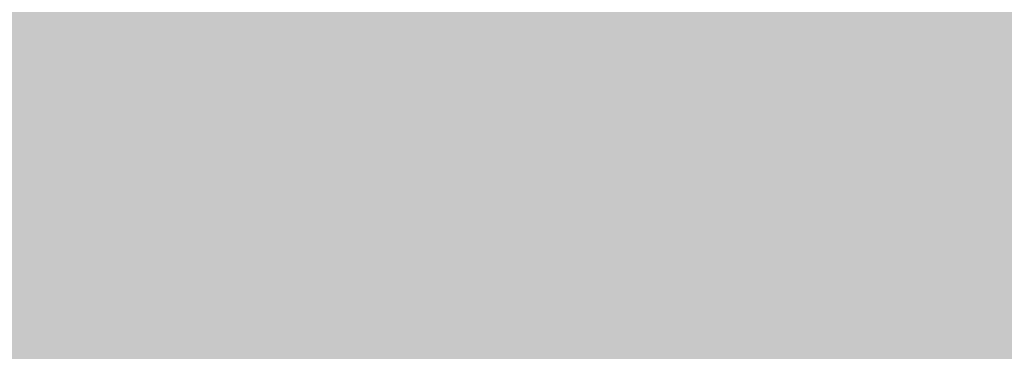
# Model space of a CAD drawing. Units: feet. Extents: x 3168 to 4724, y 827 to 1477.
# Tile 138 of 256: x 3301.129829 to 3301.134076, y 1099.01485 to 1099.016281. Entities that reach past the tile are written whole.
import ezdxf

# ---------------------------------------------------------------- set-up
doc = ezdxf.new("R2010")
doc.units = ezdxf.units.FT
doc.layers.add('A-ELEV', color=7, linetype='Continuous', lineweight=35)
doc.layers.add('A-ELEV-PATT', color=8, linetype='Continuous', lineweight=13)

msp = doc.modelspace()

# ---------------------------------------------------------------- hatches: boundary and pattern name
at = {"layer": 'A-ELEV-PATT'}
h = msp.add_hatch(color=256, dxfattribs=at)
h.dxf.hatch_style = 1
edge = h.paths.add_edge_path()
edge.add_ellipse((3552.9057615, 979.2201412), major_axis=(36.7449243, 0), ratio=0.4848484848, start_angle=0, end_angle=360)
edge = h.paths.add_edge_path()
edge.add_ellipse((3559.8916366, 929.2522824), major_axis=(36.7449243, 0), ratio=0.4848484848, start_angle=0, end_angle=360)
edge = h.paths.add_edge_path()
edge.add_line((3299.3168105, 1198.606081), (3479.9167135, 1198.606081))
edge.add_line((3479.9167135, 1198.606081), (3479.9167135, 1209.8685704))
edge.add_spline(control_points=[(3479.9167135, 1209.8685704), (3464.3011571, 1209.8685704), (3448.6856007, 1209.8685704), (3410.949139, 1209.8685704), (3388.8282339, 1209.8685704), (3355.6468761, 1209.8685704), (3344.5864235, 1209.8685704), (3327.9957446, 1209.8685704), (3322.4655183, 1209.8685704), (3314.1701788, 1209.8685704), (3311.4050657, 1209.8685704), (3307.257396, 1209.8685704), (3305.8748394, 1209.8685704), (3303.8010045, 1209.8685704), (3303.1097262, 1209.8685704), (3302.0728088, 1209.8685704), (3301.7271697, 1209.8685704), (3301.2087109, 1209.8685704), (3301.0358914, 1209.8685704), (3300.776662, 1209.8685704), (3300.6902522, 1209.8685704), (3300.5606376, 1209.8685704), (3300.5174327, 1209.8685704), (3300.4526253, 1209.8685704), (3300.4310229, 1209.8685704), (3300.3986192, 1209.8685704), (3300.387818, 1209.8685704), (3300.3662155, 1209.8685704), (3300.3456757, 1209.8685704), (3300.3455476, 1209.8685704), (3300.345505, 1209.8685704), (3300.3433041, 1209.8685704), (3300.341146, 1209.8685707), (3300.337909, 1209.8685714), (3300.33683, 1209.8685718), (3300.3339422, 1209.8685728), (3300.3321334, 1209.8685736), (3300.3255154, 1209.8685773), (3300.3207065, 1209.8685812), (3300.3109248, 1209.8685917), (3300.305952, 1209.8685984), (3300.2905113, 1209.8686233), (3300.2800452, 1209.8686461), (3300.2324255, 1209.868777), (3300.1952979, 1209.868954), (3299.9510684, 1209.8706077), (3299.7448244, 1209.8743259), (3299.4368271, 1209.8832566), (3299.3343894, 1209.8867924), (3299.181079, 1209.8929197), (3299.1300333, 1209.8950994), (3298.6522171, 1209.9168011), (3298.2294605, 1209.9457176), (3297.6016312, 1210.0023671), (3297.3934043, 1210.0234637), (3297.082652, 1210.058309), (3296.9793324, 1210.0704575), (3296.2929541, 1210.1548606), (3295.7181475, 1210.2433556), (3294.8687167, 1210.3988504), (3294.5876997, 1210.4544779), (3294.1693407, 1210.5433488), (3294.0304153, 1210.5738777), (3291.7071487, 1211.1012), (3289.6535901, 1211.8134353), (3285.7762586, 1213.5639876), (3283.9514101, 1214.6034778), (3280.512159, 1216.9800798), (3278.8972407, 1218.3175918), (3276.3799143, 1220.829489), (3275.4160415, 1221.9177379), (3274.0393421, 1223.7076996), (3273.5810428, 1224.3495346), (3273.1432283, 1225.0163162)], knot_values=[39.119033, 39.119033, 39.119033, 39.119033, 39.286353, 39.286353, 39.523379, 39.523379, 39.641892, 39.641892, 39.701148, 39.701148, 39.730777, 39.730777, 39.745591, 39.745591, 39.752998, 39.752998, 39.756701, 39.756701, 39.758553, 39.758553, 39.759479, 39.759479, 39.759942, 39.759942, 39.760173, 39.760173, 39.760289, 39.760289, 39.760405, 39.760405, 39.760463, 39.760463, 39.763389, 39.763389, 39.764851, 39.764851, 39.767304, 39.767304, 39.773825, 39.773825, 39.78057, 39.78057, 39.79477, 39.79477, 39.845194, 39.845194, 40.126715, 40.126715, 40.267476, 40.267476, 40.337856, 40.337856, 40.927023, 40.927023, 41.221606, 41.221606, 41.368898, 41.368898, 42.202622, 42.202622, 42.619485, 42.619485, 42.827916, 42.827916, 46.118323, 46.118323, 49.408731, 49.408731, 52.699139, 52.699139, 54.927489, 54.927489, 56.104228, 56.104228, 56.104228, 56.104228], weights=[1, 1, 1, 1, 1, 1, 1, 1, 1, 1, 1, 1, 1, 1, 1, 1, 1, 1, 1, 1, 1, 1, 1, 1, 1, 1, 1, 1, 1, 1, 1, 1, 1, 1, 1, 1, 1, 1, 1, 1, 1, 1, 1, 1, 1, 1, 1, 1, 1, 1, 1, 1, 1, 1, 1, 1, 1, 1, 1, 1, 1, 1, 1, 1, 1, 1, 1, 1, 1, 1, 1, 1, 1, 1], degree=3, periodic=0)
edge.add_line((3273.1432283, 1225.0163162), (3273.1432283, 1099.0163162))
edge.add_line((3273.1432283, 1099.0163162), (3299.3168105, 1099.0163162))
edge.add_line((3299.3168105, 1099.0163162), (3299.3168105, 1198.606081))
edge = h.paths.add_edge_path()
edge.add_line((3304.7584434, 1324.15806), (3479.9167135, 1324.15806))
edge.add_line((3479.9167135, 1324.15806), (3479.9167135, 1335.7146184))
edge.add_line((3479.9167135, 1335.7146184), (3269.1616284, 1335.7146184))
edge.add_spline(control_points=[(3269.1616284, 1335.7146184), (3264.0242315, 1335.7146184), (3258.364118, 1328.9581888), (3259.2643109, 1323.9002743)], knot_values=[0, 0, 0, 0, 15.412191, 15.412191, 15.412191, 15.412191], degree=3, periodic=0)
edge.add_line((3259.2643109, 1323.9002743), (3265.5168487, 1288.7691348))
edge.add_line((3265.5168487, 1288.7691348), (3275.2651026, 1261.5456259))
edge.add_line((3275.2651026, 1261.5456259), (3304.7584434, 1261.5456259))
edge.add_line((3304.7584434, 1261.5456259), (3304.7584434, 1324.15806))
h = msp.add_hatch(color=256, dxfattribs=at)
h.dxf.hatch_style = 1
h.paths.add_polyline_path([(3384.5252473, 1099.0163162), (3335.0291678, 1099.0163162), (3299.3168105, 1099.0163162), (3273.1432283, 1099.0163162), (3217.5653642, 1099.0163162), (3168.0692847, 827.1162598), (3335.0291678, 827.1162598)])

# ---------------------------------------------------------------- linework, layer by layer
at = {"layer": 'A-ELEV'}
msp.add_open_spline([(3808.5202001, 1099.0163162), (3808.5202001, 1141.413235), (3808.5202001, 1183.8101539), (3808.5202001, 1226.6353244), (3808.5202001, 1227.0635761), (3808.5202001, 1227.4918279), (3811.491871, 1248.9946729), (3814.463542, 1270.497518), (3817.4652299, 1292.2175635), (3817.4952467, 1292.434764), (3817.5252636, 1292.6519644), (3817.5728014, 1310.1067483), (3817.6203393, 1327.5615322), (3817.6678771, 1345.0163162), (3817.6678771, 1345.4579619), (3817.6678771, 1345.8996077), (3817.6678771, 1346.4560466), (3817.6678771, 1346.5708398), (3817.6678771, 1346.7528874), (3817.6678771, 1346.8201418), (3817.6678771, 1346.9348705), (3817.6678771, 1346.9823447), (3817.6678771, 1347.0385872), (3817.6678771, 1347.0473556), (3817.6678771, 1347.0736607), (3817.667877, 1347.0593025), (3817.6678766, 1347.0615455), (3817.6678764, 1347.0626669), (3817.6678754, 1347.0660311), (3817.6678743, 1347.0682738), (3817.6678701, 1347.0750012), (3817.667866, 1347.0794856), (3817.6678493, 1347.0929368), (3817.6678325, 1347.1019019), (3817.6677657, 1347.1287896), (3817.6676988, 1347.1467049), (3817.6674317, 1347.2004211), (3817.6671649, 1347.2361922), (3817.6661003, 1347.3433849), (3817.6650383, 1347.4146859), (3817.6608124, 1347.6280949), (3817.6566084, 1347.7697085), (3817.6399698, 1348.1924868), (3817.6235091, 1348.4715855), (3817.5590944, 1349.3000666), (3817.4961208, 1349.8405878), (3817.2554319, 1351.4241561), (3817.0263177, 1352.4287852), (3816.3068713, 1354.8889138), (3815.7437452, 1356.2687272), (3814.4639586, 1358.8192105), (3813.7464132, 1359.9909676), (3812.1958378, 1362.1723433), (3811.3622453, 1363.1821237), (3809.5888357, 1365.0690087), (3808.6488164, 1365.9461052), (3806.6542623, 1367.5796162), (3805.5997024, 1368.336154), (3803.3528906, 1369.7223272), (3802.1605354, 1370.352386), (3799.6008131, 1371.4535864), (3798.2326878, 1371.9254812), (3795.2800838, 1372.6346239), (3793.6931479, 1372.8720685), (3791.8694413, 1372.9264797), (3791.7408615, 1372.9292203), (3791.3533713, 1372.9341014), (3791.0927074, 1372.9329013), (3790.3041163, 1372.9150676), (3789.7695426, 1372.8841946), (3789.20919, 1372.8302363), (3789.1906217, 1372.8284241), (3789.1348916, 1372.8229123), (3789.097705, 1372.8191375), (3789.0484446, 1372.8140077), (3789.0364001, 1372.8127432), (3789.0002562, 1372.808918), (3788.9761468, 1372.8063255), (3788.9494049, 1372.8034042), (3788.9467858, 1372.8031177), (3788.9425667, 1372.8026552), (3788.9409669, 1372.8024797), (3788.9385718, 1372.8022166), (3788.9377765, 1372.8021292), (3788.9353908, 1372.8018669), (3788.8675349, 1372.7944024), (3788.7568665, 1372.7822285), (3788.7015323, 1372.7761415), (3788.5355297, 1372.7578805), (3788.4248612, 1372.7457065), (3788.092856, 1372.7091846), (3787.8715192, 1372.6848366), (3787.2075086, 1372.6117927), (3786.764835, 1372.5630968), (3785.436814, 1372.417009), (3784.5514666, 1372.3196171), (3781.8954246, 1372.0274416), (3780.1247299, 1371.8326579), (3774.8126458, 1371.2483067), (3771.2712564, 1370.8587393), (3760.6470883, 1369.6900371), (3753.5643095, 1368.9109022), (3732.3159732, 1366.5734977), (3718.1504157, 1365.015228), (3694.0067577, 1362.3593262), (3684.0286573, 1361.2616941), (3674.0505568, 1360.1640619), (3664.6006617, 1360.1640619), (3655.1507666, 1360.1640619), (3626.8010812, 1360.1640619), (3607.9012909, 1360.1640619), (3551.2019201, 1360.1640619), (3513.4023395, 1360.1640619), (3467.7251817, 1360.1640619), (3459.8476045, 1360.1640619), (3436.2148727, 1360.1640619), (3420.4597182, 1360.1640619), (3373.1942547, 1360.1640619), (3341.6839457, 1360.1640619), (3302.8481616, 1360.1640619), (3295.5226865, 1360.1640619), (3286.0382916, 1360.1640619), (3283.8793719, 1360.1640619), (3277.4026128, 1360.1640619), (3273.0847733, 1360.1640619), (3267.7328511, 1360.1640619), (3266.6987684, 1360.1640619), (3263.5965201, 1360.1640619), (3261.5283546, 1360.1640619), (3259.2369429, 1360.1640619), (3259.0136967, 1360.1640619), (3258.3439582, 1360.1640619), (3257.8974658, 1360.1640619), (3257.4309979, 1360.1640619), (3257.4110224, 1360.1640619), (3257.3705735, 1360.1640619), (3257.3754695, 1360.1640619), (3257.3745975, 1360.1640619), (3257.3739371, 1360.1640618), (3257.3719559, 1360.1640616), (3257.3706351, 1360.1640613), (3257.366673, 1360.16406), (3257.3640318, 1360.1640586), (3257.3561088, 1360.1640529), (3257.3508277, 1360.1640469), (3257.3349869, 1360.1640226), (3257.3244299, 1360.163998), (3257.2927692, 1360.1638987), (3257.2716761, 1360.1637987), (3257.208439, 1360.1633975), (3257.1663373, 1360.1629953), (3257.0402058, 1360.1613882), (3256.9563493, 1360.1597827), (3256.705504, 1360.1533932), (3256.53924, 1360.1470361), (3256.0435702, 1360.1219156), (3255.717296, 1360.0971018), (3254.7524458, 1360.0004808), (3254.1279679, 1359.906513), (3252.1800666, 1359.5253322), (3250.9415739, 1359.1439911), (3248.6701751, 1358.2432905), (3247.6357388, 1357.7238339), (3245.7326321, 1356.6034712), (3244.8633884, 1356.0020595), (3243.2531076, 1354.7428655), (3242.511972, 1354.0847309), (3240.7510518, 1352.3447812), (3239.8009609, 1351.229574), (3238.0877694, 1348.8724402), (3237.3246853, 1347.6303552), (3235.9825098, 1344.9716321), (3235.4022051, 1343.554907), (3234.5910812, 1340.8154577), (3234.3108819, 1339.5435498), (3233.9764902, 1336.8025605), (3233.9221126, 1335.3308771), (3234.1489156, 1332.5912693), (3234.3495287, 1331.3672011), (3234.7198926, 1329.9993668), (3234.7524228, 1329.8833616), (3234.853619, 1329.5347966), (3234.9258923, 1329.301685), (3235.0248359, 1329.0025524), (3235.0469235, 1328.936928), (3235.0776388, 1328.8472393), (3235.0859239, 1328.8231979), (3235.1109389, 1328.7510642), (3235.1278282, 1328.7029624), (3235.1479919, 1328.6462418), (3235.1510592, 1328.6376324), (3235.1560959, 1328.6235265), (3235.1580611, 1328.6180301), (3235.1602094, 1328.6120302), (3235.1656119, 1328.596943), (3235.1800989, 1328.556486), (3235.190263, 1328.5281009), (3235.2207556, 1328.4429457), (3235.241084, 1328.3861755), (3235.3020692, 1328.215865), (3235.3427259, 1328.1023247), (3235.4646962, 1327.7617038), (3235.5460097, 1327.5346232), (3235.7899503, 1326.8533813), (3235.9525774, 1326.39922), (3236.4404586, 1325.0367362), (3236.7657127, 1324.1284137), (3237.7414751, 1321.4034462), (3238.3919833, 1319.5868011), (3240.3435081, 1314.136866), (3241.6445245, 1310.503576), (3245.547574, 1299.6037058), (3248.149607, 1292.3371257), (3255.955706, 1270.5373853), (3261.1597719, 1256.004225), (3267.3876177, 1238.6120011), (3268.4113975, 1235.7529374), (3269.5103781, 1232.6838639), (3269.5855789, 1232.473854), (3269.7066118, 1232.1358507), (3269.752444, 1232.0078573), (3269.8273289, 1231.7987296), (3269.8563817, 1231.7175953), (3269.9063247, 1231.5781217), (3269.927215, 1231.5197823), (3269.9724682, 1231.3934057), (3269.9968311, 1231.3253685), (3270.0265026, 1231.2425062), (3270.0318112, 1231.2276812), (3270.0402823, 1231.2040243), (3270.0392242, 1231.2069792), (3270.0393595, 1231.2066014), (3270.0394271, 1231.2064125), (3270.0396301, 1231.2058458), (3270.0397654, 1231.205468), (3270.0401713, 1231.2043346), (3270.040442, 1231.2035791), (3270.041254, 1231.2013125), (3270.0417955, 1231.1998016), (3270.0434203, 1231.195269), (3270.044504, 1231.1922477), (3270.0477563, 1231.1831849), (3270.0499263, 1231.1771446), (3270.0564418, 1231.1590283), (3270.0607927, 1231.146957), (3270.0738674, 1231.1107614), (3270.0826128, 1231.0866558), (3270.1089357, 1231.0144129), (3270.1265997, 1230.9663498), (3270.1799341, 1230.8224568), (3270.2159467, 1230.7269233), (3270.3253234, 1230.4415078), (3270.4000257, 1230.2528107), (3270.6292491, 1229.6914436), (3270.7888829, 1229.3235005), (3271.2864875, 1228.2383194), (3271.6430996, 1227.5397546), (3272.7758592, 1225.515277), (3273.6141694, 1224.2605021), (3275.4160415, 1221.9177379), (3276.3799143, 1220.829489), (3278.8972407, 1218.3175918), (3280.512159, 1216.9800798), (3283.9514101, 1214.6034778), (3285.7762586, 1213.5639876), (3289.6535901, 1211.8134353), (3291.7071487, 1211.1012), (3294.0304153, 1210.5738777), (3294.1693407, 1210.5433488), (3294.5876997, 1210.4544779), (3294.8687167, 1210.3988504), (3295.7181475, 1210.2433556), (3296.2929541, 1210.1548606), (3296.9793324, 1210.0704575), (3297.082652, 1210.058309), (3297.3934043, 1210.0234637), (3297.6016312, 1210.0023671), (3298.2294605, 1209.9457176), (3298.6522171, 1209.9168011), (3299.1300333, 1209.8950994), (3299.181079, 1209.8929197), (3299.3343894, 1209.8867924), (3299.4368271, 1209.8832566), (3299.7448244, 1209.8743259), (3299.9510684, 1209.8706077), (3300.1952979, 1209.868954), (3300.2324255, 1209.868777), (3300.2800452, 1209.8686461), (3300.2905113, 1209.8686233), (3300.305952, 1209.8685984), (3300.3109248, 1209.8685917), (3300.3207065, 1209.8685812), (3300.3255154, 1209.8685773), (3300.3321334, 1209.8685736), (3300.3339422, 1209.8685728), (3300.33683, 1209.8685718), (3300.337909, 1209.8685714), (3300.341146, 1209.8685707), (3300.3433041, 1209.8685704), (3300.345505, 1209.8685704), (3300.3455476, 1209.8685704), (3300.3456757, 1209.8685704), (3300.3662155, 1209.8685704), (3300.387818, 1209.8685704), (3300.3986192, 1209.8685704), (3300.4310229, 1209.8685704), (3300.4526253, 1209.8685704), (3300.5174327, 1209.8685704), (3300.5606376, 1209.8685704), (3300.6902522, 1209.8685704), (3300.776662, 1209.8685704), (3301.0358914, 1209.8685704), (3301.2087109, 1209.8685704), (3301.7271697, 1209.8685704), (3302.0728088, 1209.8685704), (3303.1097262, 1209.8685704), (3303.8010045, 1209.8685704), (3305.8748394, 1209.8685704), (3307.257396, 1209.8685704), (3311.4050657, 1209.8685704), (3314.1701788, 1209.8685704), (3322.4655183, 1209.8685704), (3327.9957446, 1209.8685704), (3344.5864235, 1209.8685704), (3355.6468761, 1209.8685704), (3388.8282339, 1209.8685704), (3410.949139, 1209.8685704), (3477.3118546, 1209.8685704), (3521.553665, 1209.8685704), (3566.8361836, 1209.8685704), (3567.8768919, 1209.8685704), (3570.9990167, 1209.8685704), (3573.0804332, 1209.8685704), (3575.7813964, 1209.8685704), (3576.4009432, 1209.8685704), (3577.2958211, 1209.8685704), (3577.5711523, 1209.8685704), (3578.3971458, 1209.8685704), (3578.9478081, 1209.8685704), (3579.7564907, 1209.8685704), (3580.0145108, 1209.8685704), (3580.3427367, 1209.8685704), (3580.3268649, 1209.8685704), (3580.3271702, 1209.8685704), (3580.3273229, 1209.8685704), (3580.3277809, 1209.8685704), (3580.3280863, 1209.8685704), (3580.3290024, 1209.8685703), (3580.3296132, 1209.8685702), (3580.3314455, 1209.8685699), (3580.332667, 1209.8685697), (3580.336332, 1209.8685685), (3580.3387755, 1209.8685674), (3580.3461066, 1209.8685629), (3580.350995, 1209.8685584), (3580.3656627, 1209.8685402), (3580.3754446, 1209.868522), (3580.4048012, 1209.8684493), (3580.4243863, 1209.8683764), (3580.4831833, 1209.8680848), (3580.5224371, 1209.8677929), (3580.6403612, 1209.8666242), (3580.7191947, 1209.8654543), (3580.9563152, 1209.8607663), (3581.1152222, 1209.85607), (3581.5941635, 1209.8372298), (3581.9164188, 1209.8183314), (3582.8899466, 1209.7424284), (3583.547986, 1209.6661692), (3585.5318268, 1209.3606172), (3586.8672159, 1209.0538859), (3589.4715454, 1208.2524717), (3590.7402412, 1207.7578521), (3591.9954511, 1207.1588024), (3592.057809, 1207.1287398), (3592.2442418, 1207.0379536), (3592.3676757, 1206.9766317), (3592.73528, 1206.7903591), (3592.9767518, 1206.663101), (3593.2445387, 1206.5164414), (3593.2747313, 1206.4998248), (3593.3651153, 1206.4498388), (3593.4251129, 1206.4163333), (3593.6043138, 1206.3152851), (3593.7227254, 1206.2472105), (3593.8572122, 1206.1683978), (3593.8743621, 1206.1583193), (3593.925741, 1206.1280407), (3593.9598989, 1206.1077976), (3594.0620855, 1206.0468991), (3594.1298272, 1206.0060745), (3594.2084359, 1205.9581709), (3594.2196829, 1205.9513043), (3594.253391, 1205.9306863), (3594.2758193, 1205.9169166), (3594.3429716, 1205.8755358), (3594.3875633, 1205.8478526), (3594.4336161, 1205.8190499), (3594.4352559, 1205.818024), (3594.4401746, 1205.8149461), (3594.4434527, 1205.8128936), (3594.4471229, 1205.8105944), (3594.4475159, 1205.8103482), (3594.4486949, 1205.8096095), (3594.4494808, 1205.8091171), (3594.4503663, 1205.8085621), (3594.4504658, 1205.8084998), (3594.4506003, 1205.8084155), (3594.4673993, 1205.7978872), (3594.4932689, 1205.7816741), (3594.5062037, 1205.7735675), (3594.5450081, 1205.7492479), (3594.5708778, 1205.7330348), (3594.6484866, 1205.6843956), (3594.7002258, 1205.6519694), (3594.8554436, 1205.5546909), (3594.958922, 1205.4898386), (3595.2693574, 1205.2952816), (3595.4763144, 1205.1655769), (3596.0971852, 1204.7764629), (3596.5110991, 1204.5170536), (3597.7528407, 1203.7388256), (3598.5806685, 1203.220007), (3601.0641518, 1201.663551), (3602.7198073, 1200.6259137), (3607.686774, 1197.5130018), (3610.998085, 1195.4377272), (3620.9320182, 1189.2119034), (3627.5546404, 1185.0613542), (3647.4225068, 1172.6097066), (3660.6677511, 1164.3086082), (3700.403484, 1139.405313), (3726.8939725, 1122.8031161), (3757.2057154, 1103.8060516), (3761.0269697, 1101.4111839), (3764.848224, 1099.0163162), (3745.3282713, 1099.0163162), (3725.8083186, 1099.0163162), (3706.288366, 1099.0163162), (3706.288366, 1108.4532371), (3706.288366, 1117.890158), (3706.288366, 1127.3270789), (3710.7507544, 1127.3270789), (3715.2131428, 1127.3270789), (3719.6755312, 1127.3270789)], degree=3, knots=[0, 0, 0, 0, 0.982037, 0.982037, 0.991957, 0.991957, 0.991957, 1.966522, 1.966522, 1.976367, 1.976367, 1.976367, 2.976367, 2.976367, 2.976367, 3.00169, 3.00169, 3.008272, 3.008272, 3.012129, 3.012129, 3.014851, 3.014851, 3.015353, 3.015353, 3.016359, 3.016359, 3.017365, 3.017365, 3.019376, 3.019376, 3.023398, 3.023398, 3.031442, 3.031442, 3.047531, 3.047531, 3.079708, 3.079708, 3.144063, 3.144063, 3.272772, 3.272772, 3.53019, 3.53019, 4.045026, 4.045026, 5.074698, 5.074698, 6.700878, 6.700878, 8.327058, 8.327058, 9.953238, 9.953238, 11.579418, 11.579418, 13.205598, 13.205598, 14.831778, 14.831778, 16.457958, 16.457958, 18.084138, 18.084138, 18.206872, 18.206872, 18.45234, 18.45234, 18.943275, 18.943275, 18.960093, 18.960093, 18.993729, 18.993729, 19.00461, 19.00461, 19.026374, 19.026374, 19.028737, 19.028737, 19.03018, 19.03018, 19.030897, 19.030897, 19.032332, 19.032332, 19.033766, 19.033766, 19.036636, 19.036636, 19.042374, 19.042374, 19.053851, 19.053851, 19.076805, 19.076805, 19.122714, 19.122714, 19.21453, 19.21453, 19.398163, 19.398163, 19.765429, 19.765429, 20.024128, 20.024128, 20.024128, 20.092031, 20.092031, 20.227836, 20.227836, 20.499446, 20.499446, 20.556051, 20.556051, 20.66926, 20.66926, 20.895678, 20.895678, 20.948316, 20.948316, 20.963829, 20.963829, 20.994855, 20.994855, 21.002285, 21.002285, 21.017146, 21.017146, 21.01875, 21.01875, 21.021959, 21.021959, 21.022102, 21.022102, 21.022249, 21.022249, 21.022708, 21.022708, 21.023627, 21.023627, 21.025464, 21.025464, 21.029138, 21.029138, 21.036486, 21.036486, 21.051183, 21.051183, 21.080575, 21.080575, 21.139361, 21.139361, 21.256932, 21.256932, 21.492073, 21.492073, 21.962356, 21.962356, 23.01002, 23.01002, 24.057684, 24.057684, 25.105348, 25.105348, 26.153011, 26.153011, 27.776787, 27.776787, 29.400562, 29.400562, 31.024337, 31.024337, 32.278801, 32.278801, 33.533265, 33.533265, 34.467568, 34.467568, 34.553971, 34.553971, 34.726776, 34.726776, 34.775309, 34.775309, 34.793079, 34.793079, 34.82862, 34.82862, 34.834979, 34.834979, 34.839039, 34.839039, 34.839411, 34.839411, 34.840285, 34.840285, 34.842034, 34.842034, 34.845531, 34.845531, 34.852525, 34.852525, 34.866512, 34.866512, 34.894488, 34.894488, 34.950439, 34.950439, 35.062342, 35.062342, 35.286147, 35.286147, 35.733758, 35.733758, 35.821815, 35.821815, 35.828283, 35.828283, 35.832225, 35.832225, 35.834724, 35.834724, 35.836521, 35.836521, 35.838617, 35.838617, 35.839073, 35.839073, 35.839345, 35.839345, 35.839617, 35.839617, 35.840161, 35.840161, 35.841249, 35.841249, 35.843425, 35.843425, 35.847778, 35.847778, 35.856482, 35.856482, 35.873891, 35.873891, 35.908709, 35.908709, 35.978345, 35.978345, 36.117617, 36.117617, 36.396161, 36.396161, 36.953248, 36.953248, 38.067423, 38.067423, 40.295772, 40.295772, 42.524122, 42.524122, 45.81453, 45.81453, 49.104937, 49.104937, 52.395345, 52.395345, 52.603776, 52.603776, 53.020639, 53.020639, 53.854363, 53.854363, 54.001655, 54.001655, 54.296238, 54.296238, 54.885405, 54.885405, 54.955785, 54.955785, 55.096546, 55.096546, 55.378067, 55.378067, 55.42849, 55.42849, 55.442691, 55.442691, 55.449436, 55.449436, 55.455957, 55.455957, 55.458409, 55.458409, 55.459872, 55.459872, 55.462798, 55.462798, 55.462856, 55.462856, 55.462972, 55.462972, 55.463088, 55.463088, 55.463319, 55.463319, 55.463782, 55.463782, 55.464708, 55.464708, 55.46656, 55.46656, 55.470263, 55.470263, 55.47767, 55.47767, 55.492484, 55.492484, 55.522112, 55.522112, 55.581369, 55.581369, 55.699882, 55.699882, 55.936907, 55.936907, 56.410959, 56.410959, 56.42211, 56.42211, 56.444413, 56.444413, 56.451051, 56.451051, 56.454001, 56.454001, 56.459901, 56.459901, 56.462666, 56.462666, 56.463418, 56.463418, 56.464171, 56.464171, 56.465675, 56.465675, 56.468684, 56.468684, 56.474702, 56.474702, 56.486738, 56.486738, 56.51081, 56.51081, 56.558955, 56.558955, 56.655243, 56.655243, 56.847821, 56.847821, 57.232975, 57.232975, 58.003284, 58.003284, 59.543901, 59.543901, 62.625137, 62.625137, 68.787607, 68.787607, 74.950078, 74.950078, 75.27336, 75.27336, 75.919923, 75.919923, 77.213051, 77.213051, 77.377769, 77.377769, 77.707206, 77.707206, 78.366079, 78.366079, 78.462532, 78.462532, 78.655436, 78.655436, 79.041245, 79.041245, 79.105735, 79.105735, 79.234714, 79.234714, 79.492672, 79.492672, 79.502197, 79.502197, 79.521249, 79.521249, 79.523534, 79.523534, 79.528103, 79.528103, 79.528682, 79.528682, 79.528885, 79.528885, 79.529089, 79.529089, 79.529495, 79.529495, 79.530308, 79.530308, 79.531935, 79.531935, 79.535187, 79.535187, 79.541693, 79.541693, 79.554704, 79.554704, 79.580725, 79.580725, 79.632769, 79.632769, 79.736856, 79.736856, 79.94503, 79.94503, 80.361377, 80.361377, 80.421435, 80.421435, 80.421435, 81.421435, 81.421435, 81.421435, 82.421435, 82.421435, 82.421435, 83.421435, 83.421435, 83.421435, 83.421435], dxfattribs=at)

doc.saveas('drawing.dxf')
